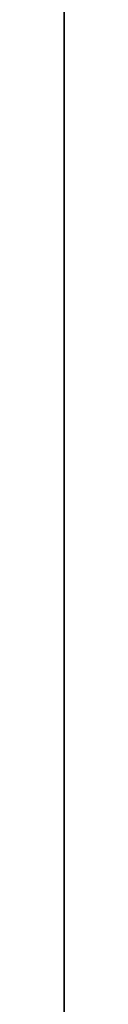
# Model space of a CAD drawing. Units: inches. Extents: x 2083 to 3317, y 1141 to 2115.
# Tile 67 of 256: x 2235.96 to 2235.96, y 1479.275 to 1481.434. Entities that reach past the tile are written whole.
import ezdxf

# ---------------------------------------------------------------- set-up
doc = ezdxf.new("R2010")
doc.units = ezdxf.units.IN
doc.layers.add('A-ANNO-DIMS', color=2, linetype='Continuous', lineweight=18)
doc.layers.add('A-WALL', color=7, linetype='Continuous', lineweight=35)
doc.layers.add('A-WALL-PATT', color=251, linetype='Continuous', lineweight=13, true_color=0x636466)
doc.styles.get("Standard").update_dxf_attribs({"font": 'arial.ttf'})
doc.dimstyles.new('ISO-25', dxfattribs={"dimtxt": 12, "dimasz": 12, "dimexe": 1.25, "dimexo": 0.625, "dimtad": 1, "dimlunit": 3, "dimtxsty": 'Standard', "dimcen": 2.5, "dimadec": 0, "dimazin": 0, "dimtfac": 1, "dimtmove": 0, "dimatfit": 3, "dimfxl": 1, "dimarcsym": 0})

# ---------------------------------------------------------------- blocks, each defined once
blk = doc.blocks.new('*D30')
at = {"layer": 'A-ANNO-DIMS', "color": 0, "lineweight": -2, "transparency": 16777216}
for p, q in [((2240.0179, 1445.2738), (2240.0179, 1448.0455)), ((2254.3293, 1445.2738), (2254.3293, 1448.0455)), ((2228.0179, 1446.7955), (2216.0179, 1446.7955)), ((2240.0179, 1446.7955), (2254.3293, 1446.7955)), ((2266.3293, 1446.7955), (2413.7649, 1446.7955))]:
    blk.add_line(p, q, dxfattribs=at)
at = {"layer": 'A-ANNO-DIMS', "color": 0, "transparency": 16777216}
for points in [[(2228.0179, 1448.7955), (2228.0179, 1444.7955), (2240.0179, 1446.7955)], [(2266.3293, 1448.7955), (2266.3293, 1444.7955), (2254.3293, 1446.7955)]]:
    blk.add_solid(points, dxfattribs=at)
at = {"layer": 'Defpoints', "color": 0, "transparency": 16777216}
for p in [(2254.3293, 1446.7955), (2240.0179, 1444.6488), (2254.3293, 1444.6488)]:
    blk.add_point(p, dxfattribs=at)
at = {"layer": 'A-ANNO-DIMS', "color": 0, "transparency": 16777216, "insert": (2346.0471, 1453.6252), "char_height": 12, "attachment_point": 5}
blk.add_mtext('WC 1\'-2 1/2" TYP.', dxfattribs=at)
blk = doc.blocks.new('*D31')
at = {"layer": 'A-ANNO-DIMS', "color": 0, "lineweight": -2, "transparency": 16777216}
for p, q in [((2237.8711, 1456.6488), (2237.8711, 1541.9152)), ((2239.3929, 1444.6488), (2236.6211, 1444.6488)), ((2237.8711, 1431.5475), (2237.8711, 1444.6488)), ((2239.3929, 1431.5475), (2236.6211, 1431.5475)), ((2237.8711, 1419.5475), (2237.8711, 1407.5475))]:
    blk.add_line(p, q, dxfattribs=at)
at = {"layer": 'A-ANNO-DIMS', "color": 0, "transparency": 16777216}
for points in [[(2235.8711, 1456.6488), (2239.8711, 1456.6488), (2237.8711, 1444.6488)], [(2235.8711, 1419.5475), (2239.8711, 1419.5475), (2237.8711, 1431.5475)]]:
    blk.add_solid(points, dxfattribs=at)
at = {"layer": 'Defpoints', "color": 0, "transparency": 16777216}
for p in [(2237.8711, 1444.6488), (2240.0179, 1444.6488), (2240.0179, 1431.5475)]:
    blk.add_point(p, dxfattribs=at)
at = {"layer": 'A-ANNO-DIMS', "color": 0, "transparency": 16777216, "insert": (2231.2175, 1505.282), "char_height": 12, "attachment_point": 5, "rotation": 90}
blk.add_mtext('1\'-1" TYP.', dxfattribs=at)
blk = doc.blocks.new('*D45')
at = {"layer": 'A-ANNO-DIMS', "color": 0, "lineweight": -2, "transparency": 16777216}
for p, q in [((2235.9598, 1478.3864), (2235.9598, 1531.3614)), ((2418.9598, 1478.3864), (2418.9598, 1531.3614)), ((2247.9598, 1530.1114), (2406.9598, 1530.1114))]:
    blk.add_line(p, q, dxfattribs=at)
at = {"layer": 'A-ANNO-DIMS', "color": 0, "transparency": 16777216}
for points in [[(2247.9598, 1532.1114), (2247.9598, 1528.1114), (2235.9598, 1530.1114)], [(2406.9598, 1532.1114), (2406.9598, 1528.1114), (2418.9598, 1530.1114)]]:
    blk.add_solid(points, dxfattribs=at)
at = {"layer": 'Defpoints', "color": 0, "transparency": 16777216}
for p in [(2418.9598, 1530.1114), (2235.9598, 1477.7614), (2418.9598, 1477.7614)]:
    blk.add_point(p, dxfattribs=at)
at = {"layer": 'A-ANNO-DIMS', "color": 0, "transparency": 16777216, "insert": (2327.4598, 1536.8673), "char_height": 12, "attachment_point": 5}
blk.add_mtext('15\'-3"', dxfattribs=at)
blk = doc.blocks.new('*D62')
at = {"layer": 'A-ANNO-DIMS', "color": 0, "lineweight": -2, "transparency": 16777216}
for p, q in [((2235.9598, 1469.3864), (2235.9598, 1522.3614)), ((2379.9598, 1469.3864), (2379.9598, 1522.3614)), ((2247.9598, 1521.1114), (2367.9598, 1521.1114))]:
    blk.add_line(p, q, dxfattribs=at)
at = {"layer": 'A-ANNO-DIMS', "color": 0, "transparency": 16777216}
for points in [[(2247.9598, 1523.1114), (2247.9598, 1519.1114), (2235.9598, 1521.1114)], [(2367.9598, 1523.1114), (2367.9598, 1519.1114), (2379.9598, 1521.1114)]]:
    blk.add_solid(points, dxfattribs=at)
at = {"layer": 'Defpoints', "color": 0, "transparency": 16777216}
for p in [(2379.9598, 1521.1114), (2235.9598, 1468.7614), (2379.9598, 1468.7614)]:
    blk.add_point(p, dxfattribs=at)
at = {"layer": 'A-ANNO-DIMS', "color": 0, "transparency": 16777216, "insert": (2307.9598, 1527.8632), "char_height": 12, "attachment_point": 5}
blk.add_mtext('12\'-0"', dxfattribs=at)

msp = doc.modelspace()

# ---------------------------------------------------------------- hatches: boundary and pattern name
at = {"layer": 'A-WALL-PATT'}
h = msp.add_hatch(color=256, dxfattribs=at)
h.dxf.hatch_style = 1
h.paths.add_polyline_path([(3126.9598, 2020.7614), (2748.9598, 2020.7614), (2604.9598, 2020.7614), (2226.9598, 2020.7614), (2226.9598, 1702.7614), (2466.9598, 1702.7614), (2466.9598, 1582.7614), (2418.9598, 1582.7614), (2418.9598, 1477.7614), (2226.9598, 1477.7614), (2226.9598, 1263.2614), (2544.9598, 1263.2614), (2544.9598, 1411.7614), (2604.9598, 1411.7614), (2685.9598, 1411.7614), (2685.9598, 1420.7614), (2604.9598, 1420.7614), (2604.9598, 1573.7614), (2604.9598, 1702.7614), (2604.9598, 2011.7614), (2748.9598, 2011.7614), (2748.9598, 1702.7614), (2862.9598, 1702.7614), (2862.9598, 1621.7614), (2871.9598, 1621.7614), (2871.9598, 1702.7614), (2883.9598, 1702.7614), (2883.9598, 1706.9395, -0.026459), (2883.9598, 1711.7614), (2757.9598, 1711.7614), (2757.9598, 1807.7614), (2787.9598, 1807.7614), (2787.9598, 1812.2614), (2757.9598, 1812.2614), (2757.9598, 2011.7614), (2877.9598, 2011.7614), (2877.9598, 1812.2614), (2847.9598, 1812.2614), (2847.9598, 1807.7614), (2889.8357, 1807.7614), (2889.8357, 1812.2614), (2882.4598, 1812.2614), (2882.4598, 2011.7614), (3117.9598, 2011.7614), (3117.9598, 1812.2614), (2937.8357, 1812.2614), (2937.8357, 1807.7614), (2995.7098, 1807.7614), (2995.7098, 1796.1177), (3000.2098, 1796.1177), (3000.2098, 1807.7614), (3117.9598, 1807.7614), (3117.9598, 1711.7614), (3000.2098, 1711.7614), (3000.2098, 1760.1177), (2998.5727, 1760.1177, -0.020711), (2995.7098, 1760.1177), (2995.7098, 1711.7614), (2931.9598, 1711.7614), (2931.9598, 1702.7614), (3126.9598, 1702.7614)])
h.paths.add_polyline_path([(2471.4598, 2011.7614), (2471.4598, 1810.0114), (2462.7169, 1810.0114), (2462.7169, 1805.5114), (2505.9598, 1805.5114), (2505.9598, 1810.0114), (2475.9598, 1810.0114), (2475.9598, 2011.7614), (2595.9598, 2011.7614), (2595.9598, 1810.0114), (2565.9598, 1810.0114), (2565.9598, 1805.5114), (2595.9598, 1805.5114), (2595.9598, 1711.7614), (2235.9598, 1711.7614), (2235.9598, 1805.5114), (2353.7098, 1805.5114), (2353.7098, 1796.0542), (2358.2098, 1796.0542), (2358.2098, 1805.5114), (2414.7169, 1805.5114), (2414.7169, 1810.0114), (2235.9598, 1810.0114), (2235.9598, 2011.7614)], flags=16)
h.paths.add_polyline_path([(2270.2047, 1994.61), (2270.2047, 1970.61), (2246.2047, 1970.61), (2246.2047, 1994.61)], flags=0)
edge = h.paths.add_edge_path(flags=0)
edge.add_ellipse((2332.0274, 1899.7982), major_axis=(-3.043, 3.043), ratio=0.168252, start_angle=-161.3322, end_angle=-156.3071, ccw=False)
edge.add_ellipse((2333.082, 1898.7435), major_axis=(-1.0546, 1.0546), ratio=0.453532, start_angle=-123.371, end_angle=-94.1591)
edge = h.paths.add_edge_path(flags=0)
edge.add_ellipse((2332.0274, 1968.8763), major_axis=(3.043, 3.043), ratio=0.168252, start_angle=18.6678, end_angle=23.6929)
edge.add_spline(control_points=[(2332.9256, 1970.6911), (2332.2268, 1970.3361), (2330.8937, 1969.6589), (2328.4131, 1970.9321), (2327.2039, 1967.7487), (2324.7096, 1969.9556), (2322.5328, 1967.0124), (2320.0128, 1971.2958), (2317.6803, 1968.1578), (2316.0405, 1967.102), (2315.4269, 1966.8096)], knot_values=[0, 0, 0, 0, 2.267059, 4.324559, 6.685584, 8.878641, 11.121502, 14.300359, 17.755284, 19.732645, 19.732645, 19.732645, 19.732645], degree=3, periodic=0)
edge.add_ellipse((2332.0274, 1968.8763), major_axis=(3.043, 3.043), ratio=0.168252, start_angle=18.6678, end_angle=23.6929, ccw=False)
edge.add_ellipse((2333.082, 1969.9309), major_axis=(1.0546, 1.0546), ratio=0.453532, start_angle=56.629, end_angle=85.8409, ccw=False)
edge = h.paths.add_edge_path(flags=0)
edge.add_spline(control_points=[(2296.4283, 1967.9879), (2293.6278, 1965.3363), (2287.7036, 1959.7271), (2299.7439, 1949.9957), (2294.5326, 1935.6685), (2290.5732, 1920.6035), (2293.3941, 1909.9737), (2296.1854, 1904.9665)], knot_values=[0.099185, 0.099185, 0.099185, 0.099185, 0.345301, 0.619822, 0.982653, 1.386093, 1.810555, 1.810555, 1.810555, 1.810555], degree=3, periodic=0)
edge.add_spline(control_points=[(2296.1854, 1904.9665), (2297.3836, 1902.6193), (2298.001, 1901.9493), (2298.553, 1901.4682)], knot_values=[0.006246, 0.006246, 0.006246, 0.006246, 0.055476, 0.055476, 0.055476, 0.055476], degree=3, periodic=0)
edge.add_spline(control_points=[(2298.553, 1901.4682), (2297.2586, 1900.9232), (2295.2253, 1900.2321), (2293.0602, 1900.6142), (2292.1014, 1900.7884), (2292.0896, 1900.7906)], knot_values=[0.312835, 0.312835, 0.312835, 0.312835, 0.40178, 0.474987, 0.475903, 0.475903, 0.475903, 0.475903], degree=3, periodic=0)
edge.add_arc((2292.7936, 1904.6641), 3.937, 215.4209, 259.6982, ccw=False)
edge.add_spline(control_points=[(2289.5853, 1902.3823), (2289.4767, 1902.5351), (2289.3685, 1902.688), (2289.2609, 1902.8412)], knot_values=[0.102872, 0.102872, 0.102872, 0.102872, 0.116896, 0.116896, 0.116896, 0.116896], degree=3, periodic=0)
edge.add_spline(control_points=[(2289.2609, 1902.8412), (2288.6866, 1902.5502), (2287.64, 1902.0199), (2285.8813, 1901.874), (2283.853, 1901.5044), (2281.72, 1899.7105), (2278.467, 1899.4929), (2276.1571, 1901.8832), (2272.259, 1899.8041), (2267.7776, 1901.8432), (2262.2439, 1900.184), (2257.4149, 1901.7821), (2254.3184, 1900.7261), (2253.1783, 1900.3373)], knot_values=[0, 0, 0, 0, 1.907977, 3.477176, 5.261074, 7.972851, 11.680248, 13.717921, 16.939592, 22.789562, 27.502503, 33.595215, 37.145618, 37.145618, 37.145618, 37.145618], degree=3, periodic=0)
edge.add_line((2253.1783, 1900.3373), (2250.2442, 1902.8412))
edge.add_line((2250.2442, 1902.8412), (2250.2442, 1965.8333))
edge.add_line((2250.2442, 1965.8333), (2253.1783, 1968.3371))
edge.add_spline(control_points=[(2253.1783, 1968.3371), (2254.3184, 1967.9483), (2257.4149, 1966.8924), (2262.2439, 1968.4904), (2267.7776, 1966.8313), (2271.5267, 1968.5372), (2273.8759, 1967.8283), (2274.2067, 1967.7276)], knot_values=[0, 0, 0, 0, 0.09018, 0.244935, 0.364644, 0.513233, 0.537855, 0.537855, 0.537855, 0.537855], degree=3, periodic=0)
edge.add_arc((2274.3529, 1963.7933), 3.937, 72.0511, 92.1279, ccw=False)
edge.add_arc((2281.2969, 1985.23), 18.5963, 252.05113, 288.56572)
edge.add_arc((2292.3167, 1956.0289), 12.6461, 71.02679, 113.77822, ccw=False)
edge = h.paths.add_edge_path(flags=0)
edge.add_spline(control_points=[(2274.8994, 1951.8562), (2275.0662, 1951.6166), (2275.2327, 1951.3766), (2275.398, 1951.1359)], knot_values=[1.409916, 1.409916, 1.409916, 1.409916, 1.43159, 1.43159, 1.43159, 1.43159], degree=3, periodic=0)
edge.add_spline(control_points=[(2275.398, 1951.1359), (2275.7921, 1950.5619), (2276.1792, 1949.9838), (2276.5455, 1949.3971)], knot_values=[1.358238, 1.358238, 1.358238, 1.358238, 1.409916, 1.409916, 1.409916, 1.409916], degree=3, periodic=0)
edge.add_line((2276.5455, 1949.3971), (2277.4373, 1947.8622))
edge.add_spline(control_points=[(2277.4373, 1947.8622), (2276.3038, 1945.6731), (2274.6397, 1942.4269), (2274.6316, 1938.0939), (2272.7991, 1930.8515), (2274.3564, 1943.897), (2275.9477, 1947.9234), (2276.5455, 1949.3971)], knot_values=[0.005632, 0.005632, 0.005632, 0.005632, 0.186014, 0.266002, 0.357087, 0.59639, 0.739732, 0.739732, 0.739732, 0.739732], degree=3, periodic=0)
edge.add_spline(control_points=[(2276.5455, 1949.3971), (2276.1792, 1949.9838), (2275.7921, 1950.5619), (2275.398, 1951.1359)], knot_values=[1.358238, 1.358238, 1.358238, 1.358238, 1.409916, 1.409916, 1.409916, 1.409916], degree=3, periodic=0)
edge.add_spline(control_points=[(2275.398, 1951.1359), (2274.9425, 1950.0805), (2274.2078, 1948.0253), (2273.9346, 1944.8515), (2272.4685, 1937.6275), (2273.4662, 1945.6965), (2274.7006, 1951.0595), (2274.8994, 1951.8562)], knot_values=[0.104364, 0.104364, 0.104364, 0.104364, 0.189636, 0.269624, 0.36071, 0.600013, 0.644622, 0.644622, 0.644622, 0.644622], degree=3, periodic=0)
h.paths.add_polyline_path([(2269.1675, 1963.1276, -0.357527), (2268.1706, 1960.9764, -0.092561), (2268.1706, 1939.4363, -0.357527), (2269.1675, 1937.2851, -0.357527), (2267.0163, 1938.282, -0.164785), (2254.6856, 1938.282, -0.357527), (2252.5344, 1937.2851, -0.357527), (2253.5313, 1939.4363, -0.092561), (2253.5313, 1960.9764, -0.357527), (2252.5344, 1963.1276, -0.357527), (2254.6856, 1962.1307, -0.164785), (2267.0163, 1962.1307, -0.357527)], flags=0)
h.paths.add_polyline_path([(2248.8741, 1967.8018), (2248.8741, 1957.0277), (2249.4578, 1957.0277), (2249.4578, 1911.6468), (2248.8741, 1911.6468), (2248.8741, 1900.8727), (2246.5119, 1900.8727, 0.197327), (2244.1497, 1902.4569), (2244.1497, 1966.2176, 0.197327), (2246.5119, 1967.8018)], flags=0)
h.paths.add_polyline_path([(2269.1675, 1931.3893, -0.357527), (2268.1706, 1929.2381, -0.092561), (2268.1706, 1907.6981, -0.357527), (2269.1675, 1905.5469, -0.357527), (2267.0163, 1906.5438, -0.164785), (2254.6856, 1906.5438, -0.357527), (2252.5344, 1905.5469, -0.357527), (2253.5313, 1907.6981, -0.092561), (2253.5313, 1929.2381, -0.357527), (2252.5344, 1931.3893, -0.357527), (2254.6856, 1930.3925, -0.164785), (2267.0163, 1930.3925, -0.357527)], flags=0)
edge = h.paths.add_edge_path(flags=0)
edge.add_spline(control_points=[(2276.1969, 1906.7237), (2276.1681, 1909.0289), (2276.114, 1913.3719), (2270.5984, 1924.925), (2273.9052, 1919.0128), (2275.9217, 1916.2621), (2275.4746, 1912.4021), (2277.2579, 1910.3806), (2276.696, 1908.225), (2276.6462, 1906.813), (2276.6178, 1906.0084)], knot_values=[0, 0, 0, 0, 8.61026, 16.221274, 18.843057, 23.804898, 27.440828, 29.356102, 31.203478, 33.650687, 33.650687, 33.650687, 33.650687], degree=3, periodic=0)
edge.add_spline(control_points=[(2276.6178, 1906.0084), (2276.6233, 1905.6241), (2276.4977, 1904.6287), (2275.4418, 1903.8547), (2274.9373, 1903.0804), (2274.8591, 1902.8412)], knot_values=[0.156488, 0.156488, 0.156488, 0.156488, 0.184398, 0.231376, 0.250598, 0.250598, 0.250598, 0.250598], degree=3, periodic=0)
edge.add_line((2274.8591, 1902.8412), (2276.506, 1902.8412))
edge.add_spline(control_points=[(2276.506, 1902.8412), (2276.7883, 1903.0849), (2277.6651, 1904.1252), (2278.2495, 1904.3407), (2277.6539, 1908.5274), (2278.1557, 1906.2278), (2278.1005, 1905.2859), (2278.8467, 1904.069), (2277.8568, 1903.4149), (2277.8742, 1902.991), (2277.9036, 1902.8412)], knot_values=[0.059574, 0.059574, 0.059574, 0.059574, 0.080753, 0.103741, 0.16972, 0.176036, 0.207137, 0.240474, 0.262341, 0.27366, 0.27366, 0.27366, 0.27366], degree=3, periodic=0)
edge.add_line((2277.9036, 1902.8412), (2280.0298, 1902.8412))
edge.add_spline(control_points=[(2280.0298, 1902.8412), (2279.8882, 1903.0884), (2279.4993, 1903.9816), (2280.1523, 1905.9393), (2278.1036, 1909.6578), (2279.7624, 1907.1853), (2280.3279, 1904.8749), (2280.4851, 1903.4896), (2281.4633, 1903.2494), (2281.7583, 1902.9365), (2281.834, 1902.8412)], knot_values=[0.013856, 0.013856, 0.013856, 0.013856, 0.034874, 0.088867, 0.107879, 0.126738, 0.158714, 0.193757, 0.217487, 0.226722, 0.226722, 0.226722, 0.226722], degree=3, periodic=0)
edge.add_spline(control_points=[(2281.834, 1902.8412), (2281.7875, 1902.8267), (2281.647, 1902.783), (2281.3955, 1902.8595), (2281.0881, 1902.9852), (2280.7207, 1903.0609), (2280.3335, 1903.0257), (2280.1248, 1902.8989), (2280.0298, 1902.8412)], knot_values=[0, 0, 0, 0, 0.14413, 0.435517, 0.749276, 1.153046, 1.548371, 1.878348, 1.878348, 1.878348, 1.878348], degree=3, periodic=0)
edge.add_line((2280.0298, 1902.8412), (2277.9036, 1902.8412))
edge.add_spline(control_points=[(2277.9036, 1902.8412), (2277.8929, 1902.7959), (2277.8654, 1902.6796), (2277.6075, 1902.6875), (2277.2741, 1902.8007), (2276.8379, 1902.6198), (2276.5838, 1902.7893), (2276.506, 1902.8412)], knot_values=[0, 0, 0, 0, 0.127189, 0.326199, 0.628009, 1.24357, 1.515331, 1.515331, 1.515331, 1.515331], degree=3, periodic=0)
edge.add_line((2276.506, 1902.8412), (2274.8591, 1902.8412))
edge.add_spline(control_points=[(2274.8591, 1902.8412), (2274.8144, 1902.8986), (2274.7251, 1903.0134), (2274.4935, 1903.119), (2274.2443, 1902.9605), (2273.9371, 1903.1849), (2273.614, 1902.9831), (2273.4083, 1902.883), (2273.3223, 1902.8412)], knot_values=[0, 0, 0, 0, 0.21843, 0.436957, 0.687977, 0.990379, 1.398396, 1.69185, 1.69185, 1.69185, 1.69185], degree=3, periodic=0)
edge.add_spline(control_points=[(2273.3223, 1902.8412), (2273.6167, 1903.4457), (2274.274, 1904.5383), (2276.0272, 1904.5737), (2276.207, 1906.5836), (2276.1969, 1906.7237)], knot_values=[0.012227, 0.012227, 0.012227, 0.012227, 0.059472, 0.106218, 0.134458, 0.134458, 0.134458, 0.134458], degree=3, periodic=0)
h.paths.add_polyline_path([(2270.7761, 1897.7898), (2270.7761, 1873.7898), (2246.7761, 1873.7898), (2246.7761, 1897.7898)], flags=0)
h.paths.add_polyline_path([(2353.7098, 1760.0051), (2353.7098, 1760.0542), (2358.2098, 1760.0542, -0.033729)], flags=0)
h.paths.add_polyline_path([(2321.8191, 1737.5292), (2341.9953, 1737.5292, -0.414214), (2343.2033, 1736.3212), (2343.2033, 1721.0206, -0.414214), (2341.9953, 1719.8127), (2321.8191, 1719.8127, -0.414214), (2320.6112, 1721.0206), (2320.6112, 1736.3212, -0.414214)], flags=0)
h.paths.add_polyline_path([(2324.235, 1736.3212), (2339.5794, 1736.3212, -0.414214), (2341.9953, 1733.9053), (2341.9953, 1725.4497, -0.414214), (2339.5794, 1723.0338), (2333.6806, 1723.0338), (2333.8453, 1722.0455, -0.870646), (2335.4254, 1721.8259, -0.767327), (2333.9227, 1721.4232), (2331.291, 1721.4232, -0.767327), (2329.7883, 1721.8259, -0.870646), (2331.3684, 1722.0455), (2331.5331, 1723.0338), (2324.235, 1723.0338, -0.414214), (2321.8191, 1725.4497), (2321.8191, 1733.9053, -0.414214)], flags=0)
h.paths.add_polyline_path([(2570.4838, 1928.6154), (2589.6838, 1928.6154), (2590.1688, 1928.6154), (2590.1688, 1904.9934), (2570.4838, 1904.9934)], flags=0)
h.paths.add_polyline_path([(2574.4473, 1927.2638, -1), (2572.8288, 1927.2638, -1)], flags=0)
h.paths.add_polyline_path([(2573.0899, 1926.9409), (2573.925, 1927.776), (2574.1477, 1927.5533), (2573.3126, 1926.7182)], flags=0)
h.paths.add_polyline_path([(2578.7791, 1919.7296, -1), (2571.5917, 1919.7296, -1)], flags=0)
h.paths.add_polyline_path([(2578.3854, 1919.7296, -1), (2571.9854, 1919.7296, -1)], flags=0)
h.paths.add_polyline_path([(2331.5958, 1729.4762, -1), (2333.618, 1729.4762, -1)], flags=0)
h.paths.add_polyline_path([(2578.0342, 1927.2638, -1), (2576.4157, 1927.2638, -1)], flags=0)
h.paths.add_polyline_path([(2576.6889, 1927.5311), (2576.9116, 1927.7538), (2577.7467, 1926.9186), (2577.524, 1926.6959)], flags=0)
h.paths.add_polyline_path([(2578.1391, 1909.8595, -1), (2572.2317, 1909.8595, -1)], flags=0)
h.paths.add_polyline_path([(2577.7454, 1909.8595, -1), (2572.6254, 1909.8595, -1)], flags=0)
h.paths.add_polyline_path([(2583.7977, 1927.2638, -1), (2582.1792, 1927.2638, -1)], flags=0)
h.paths.add_polyline_path([(2582.7186, 1927.7538), (2583.5538, 1926.9186), (2583.3311, 1926.6959), (2582.4959, 1927.5311)], flags=0)
h.paths.add_polyline_path([(2582.4959, 1927.5311), (2582.7186, 1927.7538), (2583.5538, 1926.9186), (2583.3311, 1926.6959)], flags=0)
h.paths.add_polyline_path([(2587.7391, 1920.5296, -1), (2581.8317, 1920.5296, -1)], flags=0)
h.paths.add_polyline_path([(2587.3454, 1920.5296, -1), (2582.2254, 1920.5296, -1)], flags=0)
h.paths.add_polyline_path([(2587.3846, 1927.2638, -1), (2585.7661, 1927.2638, -1)], flags=0)
h.paths.add_polyline_path([(2586.082, 1926.9802), (2586.9172, 1927.8154), (2587.1399, 1927.5927), (2586.3047, 1926.7575)], flags=0)
h.paths.add_polyline_path([(2588.3791, 1910.6595, -1), (2581.1917, 1910.6595, -1)], flags=0)
h.paths.add_polyline_path([(2587.9854, 1910.6595, -1), (2581.5854, 1910.6595, -1)], flags=0)
h.paths.add_polyline_path([(2417.1677, 1729.4779), (2437.3439, 1729.4779, -0.414214), (2438.5519, 1728.2699), (2438.5519, 1712.9693, -0.414214), (2437.3439, 1711.7614), (2417.1677, 1711.7614, -0.414214), (2415.9598, 1712.9693), (2415.9598, 1728.2699, -0.414214)], flags=0)
h.paths.add_polyline_path([(2419.5836, 1728.2699), (2434.928, 1728.2699, -0.414214), (2437.3439, 1725.8541), (2437.3439, 1717.3984, -0.414214), (2434.928, 1714.9825), (2429.0292, 1714.9825), (2429.1939, 1713.9942, -0.870646), (2430.774, 1713.7746, -0.767327), (2429.2713, 1713.372), (2426.6396, 1713.372, -0.767327), (2425.1369, 1713.7746, -0.870646), (2426.717, 1713.9942), (2426.8817, 1714.9825), (2419.5836, 1714.9825, -0.414214), (2417.1677, 1717.3984), (2417.1677, 1725.8541, -0.414214)], flags=0)
h.paths.add_polyline_path([(2419.5836, 1728.2699), (2434.928, 1728.2699, -0.414214), (2437.3439, 1725.8541), (2437.3439, 1717.3984, -0.414214), (2434.928, 1714.9825), (2429.0292, 1714.9825), (2428.3581, 1719.009), (2427.5528, 1719.009), (2426.8817, 1714.9825), (2419.5836, 1714.9825, -0.414214), (2417.1677, 1717.3984), (2417.1677, 1725.8541, -0.414214)], flags=0)
h.paths.add_polyline_path([(2426.9444, 1721.4249, -1), (2428.9666, 1721.4249, -1)], flags=0)
h.paths.add_polyline_path([(2475.9598, 1702.7614), (2595.9598, 1702.7614), (2595.9598, 1582.7614), (2475.9598, 1582.7614)], flags=16)
h.paths.add_polyline_path([(2427.9598, 1573.7614), (2595.9598, 1573.7614), (2595.9598, 1468.7614), (2595.9598, 1420.7614), (2384.4598, 1420.7614), (2384.4598, 1468.7614), (2427.9598, 1468.7614)], flags=16)
h.paths.add_polyline_path([(2379.9598, 1468.7614), (2379.9598, 1420.7614), (2235.9598, 1420.7614), (2235.9598, 1468.7614)], flags=16)
h.paths.add_polyline_path([(2317.816, 1466.6958), (2337.9922, 1466.6958, -0.414214), (2339.2002, 1465.4878), (2339.2002, 1450.1872, -0.414214), (2337.9922, 1448.9792), (2317.816, 1448.9792, -0.414214), (2316.6081, 1450.1872), (2316.6081, 1465.4878, -0.414214)], flags=0)
h.paths.add_polyline_path([(2320.2319, 1465.4878), (2335.5763, 1465.4878, -0.414214), (2337.9922, 1463.0719), (2337.9922, 1454.6163, -0.414214), (2335.5763, 1452.2004), (2329.6775, 1452.2004), (2329.8422, 1451.212, -0.870646), (2331.4223, 1450.9925, -0.767327), (2329.9196, 1450.5898), (2327.2879, 1450.5898, -0.767327), (2325.7852, 1450.9925, -0.870646), (2327.3653, 1451.212), (2327.53, 1452.2004), (2320.2319, 1452.2004, -0.414214), (2317.816, 1454.6163), (2317.816, 1463.0719, -0.414214)], flags=0)
h.paths.add_polyline_path([(2320.2319, 1465.4878), (2335.5763, 1465.4878, -0.414214), (2337.9922, 1463.0719), (2337.9922, 1454.6163, -0.414214), (2335.5763, 1452.2004), (2329.6775, 1452.2004), (2329.0064, 1456.2269), (2328.2011, 1456.2269), (2327.53, 1452.2004), (2320.2319, 1452.2004, -0.414214), (2317.816, 1454.6163), (2317.816, 1463.0719, -0.414214)], flags=0)
h.paths.add_polyline_path([(2327.5926, 1458.6428, -1), (2329.6148, 1458.6428, -1)], flags=0)
h.paths.add_polyline_path([(2244.4117, 1433.3405), (2241.9209, 1433.3405, -0.414214), (2240.0179, 1435.2435), (2240.0179, 1440.9528, -0.414211), (2241.9209, 1442.8559), (2244.4117, 1442.8559, -1.976472)], flags=0)
h.paths.add_polyline_path([(2245.3569, 1434.3975, -0.414214), (2245.3569, 1441.7988, -2.144098)], flags=0)
h.paths.add_polyline_path([(2535.9598, 1416.2614), (2535.9598, 1272.2614), (2235.9598, 1272.2614), (2235.9598, 1416.2614)], flags=16)
h.paths.add_polyline_path([(2260.1196, 1384.2928), (2260.1196, 1362.0386), (2237.8654, 1362.0386), (2237.8654, 1384.2928)], flags=0)
edge = h.paths.add_edge_path(flags=0)
edge.add_line((2318.2518, 1362.0933), (2318.1458, 1362.001))
edge.add_ellipse((2317.4451, 1360.431), major_axis=(2.8216, 2.8216), ratio=0.168252, start_angle=18.6678, end_angle=20.9481, ccw=False)
edge.add_ellipse((2318.423, 1361.409), major_axis=(0.9779, 0.9779), ratio=0.453532, start_angle=56.629, end_angle=70.2262, ccw=False)
edge = h.paths.add_edge_path(flags=0)
edge.add_line((2319.1074, 1295.5711), (2319.015, 1295.6771))
edge.add_ellipse((2317.4451, 1296.3778), major_axis=(-2.8216, 2.8216), ratio=0.168252, start_angle=-161.3322, end_angle=-159.0519, ccw=False)
edge.add_ellipse((2318.423, 1295.3999), major_axis=(-0.9779, 0.9779), ratio=0.453532, start_angle=-123.371, end_angle=-109.7738)
edge = h.paths.add_edge_path(flags=0)
edge.add_spline(control_points=[(2284.2103, 1301.1702), (2284.5807, 1300.4447), (2284.8912, 1299.892), (2285.1596, 1299.461)], knot_values=[0.039066, 0.039066, 0.039066, 0.039066, 0.055476, 0.055476, 0.055476, 0.055476], degree=3, periodic=0)
edge.add_line((2285.1596, 1299.461), (2284.2103, 1301.1702))
edge = h.paths.add_edge_path(flags=0)
edge.add_line((2280.4125, 1297.298), (2283.37, 1297.0361))
edge.add_line((2283.37, 1297.0361), (2286.4057, 1297.9263))
edge.add_spline(control_points=[(2286.4057, 1297.9263), (2285.3055, 1297.4631), (2284.3448, 1297.1292), (2283.37, 1297.0361)], knot_values=[0.394369, 0.394369, 0.394369, 0.394369, 0.475903, 0.475903, 0.475903, 0.475903], degree=3, periodic=0)
edge.add_spline(control_points=[(2283.37, 1297.0361), (2283.2814, 1297.0277), (2282.3163, 1296.9573), (2281.3125, 1297.1345), (2280.4234, 1297.296), (2280.4125, 1297.298)], knot_values=[0.312835, 0.312835, 0.312835, 0.312835, 0.320246, 0.393453, 0.394369, 0.394369, 0.394369, 0.394369], degree=3, periodic=0)
edge = h.paths.add_edge_path(flags=0)
edge.add_line((2284.4356, 1359.6073), (2280.4463, 1355.328))
edge.add_line((2280.4463, 1355.328), (2279.58, 1351.0178))
edge.add_line((2279.58, 1351.0178), (2282.413, 1346.5804))
edge.add_spline(control_points=[(2282.413, 1346.5804), (2283.1533, 1345.5892), (2284.2529, 1344.0289), (2284.801, 1342.3872), (2284.9352, 1341.8055)], knot_values=[1.240098, 1.240098, 1.240098, 1.240098, 1.332892, 1.382712, 1.382712, 1.382712, 1.382712], degree=3, periodic=0)
edge.add_spline(control_points=[(2284.9352, 1341.8055), (2285.3191, 1340.1406), (2285.233, 1338.4092), (2284.9099, 1336.6541)], knot_values=[1.097484, 1.097484, 1.097484, 1.097484, 1.240098, 1.240098, 1.240098, 1.240098], degree=3, periodic=0)
edge.add_spline(control_points=[(2284.9099, 1336.6541), (2284.5868, 1334.899), (2284.0267, 1333.1203), (2283.4626, 1331.3606)], knot_values=[0.95487, 0.95487, 0.95487, 0.95487, 1.097484, 1.097484, 1.097484, 1.097484], degree=3, periodic=0)
edge.add_line((2283.4626, 1331.3606), (2281.8904, 1326.1534))
edge.add_line((2281.8904, 1326.1534), (2280.7563, 1321.0561))
edge.add_line((2280.7563, 1321.0561), (2280.2992, 1316.002))
edge.add_line((2280.2992, 1316.002), (2280.7159, 1310.9501))
edge.add_line((2280.7159, 1310.9501), (2282.0281, 1305.9721))
edge.add_line((2282.0281, 1305.9721), (2284.2103, 1301.1702))
edge.add_spline(control_points=[(2284.2103, 1301.1702), (2283.3407, 1302.7302), (2282.6119, 1304.3365), (2282.0281, 1305.9721)], knot_values=[0.099185, 0.099185, 0.099185, 0.099185, 0.241799, 0.241799, 0.241799, 0.241799], degree=3, periodic=0)
edge.add_spline(control_points=[(2282.0281, 1305.9721), (2281.4443, 1307.6078), (2281.0055, 1309.2728), (2280.7159, 1310.9501)], knot_values=[0.241799, 0.241799, 0.241799, 0.241799, 0.384413, 0.384413, 0.384413, 0.384413], degree=3, periodic=0)
edge.add_spline(control_points=[(2280.7159, 1310.9501), (2280.4332, 1312.5876), (2280.2894, 1314.277), (2280.2989, 1315.962), (2280.2992, 1316.002)], knot_values=[0.384413, 0.384413, 0.384413, 0.384413, 0.523647, 0.527028, 0.527028, 0.527028, 0.527028], degree=3, periodic=0)
edge.add_spline(control_points=[(2280.2992, 1316.002), (2280.3123, 1317.687), (2280.4779, 1319.3679), (2280.7563, 1321.0561)], knot_values=[0.527028, 0.527028, 0.527028, 0.527028, 0.669642, 0.669642, 0.669642, 0.669642], degree=3, periodic=0)
edge.add_spline(control_points=[(2280.7563, 1321.0561), (2281.0346, 1322.7443), (2281.4259, 1324.4396), (2281.8904, 1326.1534)], knot_values=[0.669642, 0.669642, 0.669642, 0.669642, 0.812256, 0.812256, 0.812256, 0.812256], degree=3, periodic=0)
edge.add_spline(control_points=[(2281.8904, 1326.1534), (2282.2644, 1327.5333), (2282.7879, 1329.2618), (2283.3528, 1331.0178), (2283.4626, 1331.3606)], knot_values=[0.812256, 0.812256, 0.812256, 0.812256, 0.927087, 0.95487, 0.95487, 0.95487, 0.95487], degree=3, periodic=0)
edge.add_line((2283.4626, 1331.3606), (2284.9099, 1336.6541))
edge.add_line((2284.9099, 1336.6541), (2284.9352, 1341.8055))
edge.add_line((2284.9352, 1341.8055), (2282.413, 1346.5804))
edge.add_spline(control_points=[(2282.413, 1346.5804), (2281.2751, 1348.1038), (2280.0784, 1349.5703), (2279.58, 1351.0178)], knot_values=[1.382712, 1.382712, 1.382712, 1.382712, 1.525326, 1.525326, 1.525326, 1.525326], degree=3, periodic=0)
edge.add_spline(control_points=[(2279.58, 1351.0178), (2279.4433, 1351.4147), (2279.1363, 1352.8569), (2279.7352, 1354.2904), (2280.4463, 1355.328)], knot_values=[1.525326, 1.525326, 1.525326, 1.525326, 1.564439, 1.667941, 1.667941, 1.667941, 1.667941], degree=3, periodic=0)
edge.add_spline(control_points=[(2280.4463, 1355.328), (2281.4261, 1356.7578), (2282.9308, 1358.1826), (2284.4356, 1359.6073)], knot_values=[1.667941, 1.667941, 1.667941, 1.667941, 1.810555, 1.810555, 1.810555, 1.810555], degree=3, periodic=0)
edge.add_arc((2280.6231, 1348.5182), 11.7262, 71.02679, 113.77822)
edge.add_arc((2270.4049, 1375.5952), 17.2436, 252.05113, 288.56572, ccw=False)
edge.add_arc((2263.966, 1355.7178), 3.6506, 72.0511, 92.1279)
edge.add_arc((2263.966, 1355.7178), 3.6506, 92.1279, 177.9851)
edge.add_spline(control_points=[(2260.3176, 1355.8462), (2260.2604, 1354.2207), (2260.5513, 1350.1865), (2262.9993, 1346.7663), (2264.4727, 1344.649)], knot_values=[1.43159, 1.43159, 1.43159, 1.43159, 1.564144, 1.770695, 1.770695, 1.770695, 1.770695], degree=3, periodic=0)
edge.add_line((2264.4727, 1344.649), (2264.9356, 1343.9825))
edge.add_spline(control_points=[(2263.801, 1340.2481), (2263.8432, 1340.5141), (2264.0672, 1341.7565), (2264.5127, 1343.0025), (2264.935, 1343.9811)], knot_values=[0.53657, 0.53657, 0.53657, 0.53657, 0.559349, 0.644622, 0.644622, 0.644622, 0.644622], degree=3, periodic=0)
edge.add_spline(control_points=[(2264.935, 1343.9811), (2265.1178, 1343.715), (2265.2989, 1343.4479), (2265.4768, 1343.1794)], knot_values=[1.384077, 1.384077, 1.384077, 1.384077, 1.409916, 1.409916, 1.409916, 1.409916], degree=3, periodic=0)
edge.add_spline(control_points=[(2265.4768, 1343.1794), (2265.6546, 1342.9108), (2265.8293, 1342.6408), (2265.9991, 1342.3688)], knot_values=[1.358238, 1.358238, 1.358238, 1.358238, 1.384077, 1.384077, 1.384077, 1.384077], degree=3, periodic=0)
edge.add_line((2265.9991, 1342.3688), (2266.826, 1340.9455))
edge.add_spline(control_points=[(2266.826, 1340.9455), (2268.8944, 1337.0897), (2271.3982, 1325.843), (2270.5162, 1310.5686), (2275.9194, 1301.8606), (2277.7895, 1299.1994)], knot_values=[0.116896, 0.116896, 0.116896, 0.116896, 0.472987, 1.050969, 1.313793, 1.313793, 1.313793, 1.313793], degree=3, periodic=0)
edge.add_spline(control_points=[(2277.7895, 1299.1994), (2277.8394, 1299.1285), (2277.8894, 1299.0575), (2277.9396, 1298.9866)], knot_values=[0.109884, 0.109884, 0.109884, 0.109884, 0.116896, 0.116896, 0.116896, 0.116896], degree=3, periodic=0)
edge.add_line((2277.9396, 1298.9866), (2277.7888, 1299.1991))
edge.add_spline(control_points=[(2277.7888, 1299.1991), (2277.2566, 1298.9294), (2276.2864, 1298.4379), (2275.0394, 1298.3344), (2274.3833, 1298.2389), (2274.2153, 1298.2093)], knot_values=[33.12187, 33.12187, 33.12187, 33.12187, 35.029056, 36.598255, 37.144827, 37.144827, 37.144827, 37.144827], degree=3, periodic=0)
edge.add_line((2274.2153, 1298.2093), (2273.0731, 1297.893))
edge.add_spline(control_points=[(2273.0731, 1297.893), (2272.3229, 1297.5798), (2271.0392, 1296.5105), (2269.2484, 1296.2261), (2268.4231, 1296.3747)], knot_values=[26.532584, 26.532584, 26.532584, 26.532584, 29.198919, 31.839101, 31.839101, 31.839101, 31.839101], degree=3, periodic=0)
edge.add_line((2268.4231, 1296.3747), (2263.8785, 1297.4575))
edge.add_spline(control_points=[(2263.8785, 1297.4575), (2263.5561, 1297.3594), (2261.8603, 1296.8387), (2260.2388, 1297.2824), (2258.9335, 1297.5165)], knot_values=[15.919551, 15.919551, 15.919551, 15.919551, 16.939592, 21.226067, 21.226067, 21.226067, 21.226067], degree=3, periodic=0)
edge.add_line((2258.9335, 1297.5165), (2254.0552, 1297.329))
edge.add_spline(control_points=[(2254.0552, 1297.329), (2253.7555, 1297.2958), (2252.1137, 1297.1652), (2250.4619, 1297.5442), (2249.1297, 1297.6679)], knot_values=[5.306517, 5.306517, 5.306517, 5.306517, 6.276435, 10.613034, 10.613034, 10.613034, 10.613034], degree=3, periodic=0)
edge.add_line((2249.1297, 1297.6679), (2244.3316, 1296.8778))
edge.add_line((2244.3316, 1296.8778), (2241.611, 1299.1994))
edge.add_line((2241.611, 1299.1994), (2241.611, 1357.6094))
edge.add_line((2241.611, 1357.6094), (2244.3316, 1359.9311))
edge.add_line((2244.3316, 1359.9311), (2252.7288, 1359.5427))
edge.add_spline(control_points=[(2252.7288, 1359.5427), (2252.8709, 1359.5464), (2253.3057, 1359.5482), (2253.7398, 1359.5143), (2254.0317, 1359.4824)], knot_values=[0.233291, 0.233291, 0.233291, 0.233291, 0.244935, 0.268927, 0.268927, 0.268927, 0.268927], degree=3, periodic=0)
edge.add_line((2254.0317, 1359.4824), (2259.5872, 1359.4164))
edge.add_spline(control_points=[(2259.5872, 1359.4164), (2260.6771, 1359.6285), (2262.0732, 1359.897), (2263.5237, 1359.4593), (2263.8304, 1359.366)], knot_values=[0.422516, 0.422516, 0.422516, 0.422516, 0.513233, 0.537855, 0.537855, 0.537855, 0.537855], degree=3, periodic=0)
edge.add_arc((2263.966, 1355.7178), 3.6506, 72.0511, 92.1279, ccw=False)
edge.add_arc((2270.4049, 1375.5952), 17.2436, 252.05113, 288.56572)
edge.add_arc((2280.6231, 1348.5182), 11.7262, 71.02679, 113.77822, ccw=False)
h.paths.add_polyline_path([(2240.3405, 1359.4347), (2240.3405, 1349.4444), (2240.8818, 1349.4444), (2240.8818, 1307.3645), (2240.3405, 1307.3645), (2240.3405, 1297.3741), (2238.1502, 1297.3741, 0.197327), (2235.9598, 1298.8431), (2235.9598, 1357.9657, 0.197327), (2238.1502, 1359.4347)], flags=0)
h.paths.add_polyline_path([(2259.1578, 1355.1005, -0.357527), (2258.2334, 1353.1058, -0.092561), (2258.2334, 1333.1326, -0.357527), (2259.1578, 1331.1379, -0.357527), (2257.1631, 1332.0622, -0.164785), (2245.7293, 1332.0622, -0.357527), (2243.7346, 1331.1379, -0.357527), (2244.6589, 1333.1326, -0.092561), (2244.6589, 1353.1058, -0.357527), (2243.7346, 1355.1005, -0.357527), (2245.7293, 1354.1761, -0.164785), (2257.1631, 1354.1761, -0.357527)], flags=0)
edge = h.paths.add_edge_path(flags=0)
edge.add_line((2265.9991, 1342.3688), (2266.826, 1340.9455))
edge.add_line((2266.826, 1340.9455), (2265.3076, 1337.8141))
edge.add_line((2265.3076, 1337.8141), (2264.3582, 1334.6529))
edge.add_line((2264.3582, 1334.6529), (2264.262, 1333.7997))
edge.add_spline(control_points=[(2264.262, 1333.7997), (2264.2084, 1333.1871), (2264.1621, 1332.3655), (2264.0071, 1331.4139), (2263.969, 1331.2018)], knot_values=[0.464444, 0.464444, 0.464444, 0.464444, 0.516691, 0.531608, 0.531608, 0.531608, 0.531608], degree=3, periodic=0)
edge.add_spline(control_points=[(2263.969, 1331.2018), (2263.7745, 1330.1189), (2263.4244, 1328.7908), (2263.2574, 1328.5307), (2263.234, 1328.5146)], knot_values=[0.372682, 0.372682, 0.372682, 0.372682, 0.44885, 0.464444, 0.464444, 0.464444, 0.464444], degree=3, periodic=0)
edge.add_spline(control_points=[(2263.234, 1328.5146), (2263.0964, 1328.4202), (2263.1312, 1329.3015), (2263.275, 1330.6157)], knot_values=[0.280919, 0.280919, 0.280919, 0.280919, 0.372682, 0.372682, 0.372682, 0.372682], degree=3, periodic=0)
edge.add_spline(control_points=[(2263.275, 1330.6157), (2263.4187, 1331.93), (2263.6715, 1333.6773), (2263.9699, 1335.315)], knot_values=[0.189157, 0.189157, 0.189157, 0.189157, 0.280919, 0.280919, 0.280919, 0.280919], degree=3, periodic=0)
edge.add_spline(control_points=[(2263.9699, 1335.315), (2264.1005, 1336.0322), (2264.4188, 1337.6219), (2264.7548, 1338.8644), (2264.9474, 1339.4911)], knot_values=[0.097394, 0.097394, 0.097394, 0.097394, 0.137578, 0.189157, 0.189157, 0.189157, 0.189157], degree=3, periodic=0)
edge.add_spline(control_points=[(2264.9474, 1339.4911), (2265.29, 1340.6061), (2265.6442, 1341.494), (2265.9991, 1342.3688)], knot_values=[0.005632, 0.005632, 0.005632, 0.005632, 0.097394, 0.097394, 0.097394, 0.097394], degree=3, periodic=0)
h.paths.add_polyline_path([(2259.1578, 1325.671, -0.357527), (2258.2334, 1323.6763, -0.092561), (2258.2334, 1303.7031, -0.357527), (2259.1578, 1301.7084, -0.357527), (2257.1631, 1302.6327, -0.164785), (2245.7293, 1302.6327, -0.357527), (2243.7346, 1301.7084, -0.357527), (2244.6589, 1303.7031, -0.092561), (2244.6589, 1323.6763, -0.357527), (2243.7346, 1325.671, -0.357527), (2245.7293, 1324.7466, -0.164785), (2257.1631, 1324.7466, -0.357527)], flags=0)
edge = h.paths.add_edge_path(flags=0)
edge.add_spline(control_points=[(2261.7089, 1317.3114), (2261.6795, 1317.4176), (2261.7619, 1317.3885), (2262.4907, 1316.0899), (2262.9622, 1315.3009)], knot_values=[14.955861, 14.955861, 14.955861, 14.955861, 16.221274, 18.694826, 18.694826, 18.694826, 18.694826], degree=3, periodic=0)
edge.add_spline(control_points=[(2262.9622, 1315.3009), (2262.9904, 1315.2536), (2263.7021, 1314.0674), (2264.349, 1313.1272), (2264.7301, 1312.1642)], knot_values=[18.694826, 18.694826, 18.694826, 18.694826, 18.843057, 22.433791, 22.433791, 22.433791, 22.433791], degree=3, periodic=0)
edge.add_spline(control_points=[(2264.7301, 1312.1642), (2264.8756, 1311.7964), (2265.1769, 1310.7698), (2265.1431, 1309.5593), (2265.2477, 1308.8242)], knot_values=[22.433791, 22.433791, 22.433791, 22.433791, 23.804898, 26.172756, 26.172756, 26.172756, 26.172756], degree=3, periodic=0)
edge.add_line((2265.2477, 1308.8242), (2265.8508, 1307.1719))
edge.add_spline(control_points=[(2265.8508, 1307.1719), (2266.065, 1306.8217), (2266.3844, 1306.3322), (2266.4244, 1305.7805), (2266.4204, 1305.6112)], knot_values=[28.062562, 28.062562, 28.062562, 28.062562, 29.356102, 29.911721, 29.911721, 29.911721, 29.911721], degree=3, periodic=0)
edge.add_spline(control_points=[(2266.4204, 1305.6112), (2266.4161, 1305.4326), (2266.394, 1305.25), (2266.3648, 1305.0659)], knot_values=[29.911721, 29.911721, 29.911721, 29.911721, 30.497837, 30.497837, 30.497837, 30.497837], degree=3, periodic=0)
edge.add_line((2266.3648, 1305.0659), (2266.0662, 1302.1363))
edge.add_spline(control_points=[(2266.0662, 1302.1363), (2266.0712, 1301.78), (2265.9981, 1301.2), (2265.6633, 1300.759), (2265.5089, 1300.5859)], knot_values=[0.156488, 0.156488, 0.156488, 0.156488, 0.184398, 0.203543, 0.203543, 0.203543, 0.203543], degree=3, periodic=0)
edge.add_line((2265.5089, 1300.5859), (2264.4353, 1299.1994))
edge.add_line((2264.4353, 1299.1994), (2265.9624, 1299.1994))
edge.add_line((2265.9624, 1299.1994), (2267.336, 1301.1753))
edge.add_line((2267.336, 1301.1753), (2267.3117, 1301.9862))
edge.add_spline(control_points=[(2267.3117, 1301.9862), (2267.2611, 1302.8624), (2267.1602, 1303.7371), (2267.2715, 1303.3259)], knot_values=[0.126229, 0.126229, 0.126229, 0.126229, 0.166617, 0.166617, 0.166617, 0.166617], degree=3, periodic=0)
edge.add_spline(control_points=[(2267.2715, 1303.3259), (2267.28, 1303.2943), (2267.3098, 1303.1754), (2267.3735, 1302.8836), (2267.4061, 1302.6828), (2267.4179, 1302.601)], knot_values=[0.166617, 0.166617, 0.166617, 0.166617, 0.16972, 0.176036, 0.180765, 0.180765, 0.180765, 0.180765], degree=3, periodic=0)
edge.add_spline(control_points=[(2267.7439, 1300.9875), (2267.6876, 1301.1509), (2267.4805, 1301.6567), (2267.4838, 1302.1448), (2267.4179, 1302.601)], knot_values=[0.180765, 0.180765, 0.180765, 0.180765, 0.193767, 0.220139, 0.220139, 0.220139, 0.220139], degree=3, periodic=0)
edge.add_line((2267.4179, 1302.601), (2267.7439, 1300.9875))
edge.add_spline(control_points=[(2267.7439, 1300.9875), (2267.832, 1300.7319), (2267.932, 1300.3099), (2267.5548, 1299.9745), (2267.4294, 1299.8292)], knot_values=[0.220139, 0.220139, 0.220139, 0.220139, 0.240474, 0.25489, 0.25489, 0.25489, 0.25489], degree=3, periodic=0)
edge.add_line((2267.4294, 1299.8292), (2267.2584, 1299.1994))
edge.add_line((2267.2584, 1299.1994), (2269.23, 1299.1994))
edge.add_spline(control_points=[(2269.23, 1299.1994), (2269.0987, 1299.4287), (2268.8428, 1300.0163), (2269.0116, 1300.9159), (2268.9468, 1301.6607)], knot_values=[0.013856, 0.013856, 0.013856, 0.013856, 0.034874, 0.067073, 0.067073, 0.067073, 0.067073], degree=3, periodic=0)
edge.add_line((2268.9468, 1301.6607), (2268.4316, 1303.6031))
edge.add_spline(control_points=[(2268.4316, 1303.6031), (2268.1756, 1304.1924), (2267.5962, 1305.2513), (2268.0407, 1304.6232), (2268.2514, 1304.2824)], knot_values=[0.090155, 0.090155, 0.090155, 0.090155, 0.107879, 0.120289, 0.120289, 0.120289, 0.120289], degree=3, periodic=0)
edge.add_spline(control_points=[(2268.2514, 1304.2824), (2268.3609, 1304.1053), (2269.0578, 1302.918), (2269.3827, 1301.5904), (2269.5214, 1300.7759), (2269.5752, 1300.5558)], knot_values=[0.120289, 0.120289, 0.120289, 0.120289, 0.126738, 0.158714, 0.173506, 0.173506, 0.173506, 0.173506], degree=3, periodic=0)
edge.add_line((2269.5752, 1300.5558), (2270.6858, 1299.4213))
edge.add_spline(control_points=[(2270.6858, 1299.4213), (2270.7672, 1299.3573), (2270.8379, 1299.2814), (2270.9029, 1299.1994)], knot_values=[0.21816, 0.21816, 0.21816, 0.21816, 0.226722, 0.226722, 0.226722, 0.226722], degree=3, periodic=0)
edge.add_line((2270.9372, 1299.1929), (2270.9029, 1299.1994))
edge.add_spline(control_points=[(2270.9029, 1299.1994), (2270.8598, 1299.186), (2270.7295, 1299.1455), (2270.4963, 1299.2164), (2270.2717, 1299.3083), (2270.121, 1299.348), (2270.0633, 1299.3596)], knot_values=[0.939174, 0.939174, 0.939174, 0.939174, 1.083304, 1.374691, 1.68845, 1.878348, 1.878348, 1.878348, 1.878348], degree=3, periodic=0)
edge.add_line((2270.0633, 1299.3596), (2269.23, 1299.1994))
edge.add_line((2269.23, 1299.1994), (2267.2584, 1299.1994))
edge.add_spline(control_points=[(2267.2584, 1299.1994), (2267.2484, 1299.1574), (2267.223, 1299.0497), (2266.9838, 1299.0569), (2266.8092, 1299.1162), (2266.6769, 1299.1091), (2266.6365, 1299.1048)], knot_values=[0.757665, 0.757665, 0.757665, 0.757665, 0.884854, 1.083864, 1.385675, 1.515331, 1.515331, 1.515331, 1.515331], degree=3, periodic=0)
edge.add_spline(control_points=[(2266.6365, 1299.1048), (2266.4852, 1299.0888), (2266.2358, 1299.0171), (2266.0346, 1299.1513), (2265.9624, 1299.1994)], knot_values=[0, 0, 0, 0, 0.485905, 0.757665, 0.757665, 0.757665, 0.757665], degree=3, periodic=0)
edge.add_line((2265.9624, 1299.1994), (2264.4353, 1299.1994))
edge.add_line((2264.4353, 1299.1994), (2263.8584, 1299.3671))
edge.add_spline(control_points=[(2263.8584, 1299.3671), (2263.8189, 1299.3709), (2263.7795, 1299.3857), (2263.7401, 1299.4015)], knot_values=[0.845925, 0.845925, 0.845925, 0.845925, 0.978627, 0.978627, 0.978627, 0.978627], degree=3, periodic=0)
edge.add_line((2263.7218, 1299.3964), (2263.0103, 1299.1994))
edge.add_spline(control_points=[(2263.0103, 1299.1994), (2263.2458, 1299.6829), (2263.506, 1300.1281), (2263.8735, 1300.408)], knot_values=[0.012227, 0.012227, 0.012227, 0.012227, 0.052971, 0.052971, 0.052971, 0.052971], degree=3, periodic=0)
edge.add_spline(control_points=[(2263.8735, 1300.408), (2263.9321, 1300.4527), (2264.0842, 1300.553), (2264.2552, 1300.6242), (2264.3597, 1300.6647)], knot_values=[0.052971, 0.052971, 0.052971, 0.052971, 0.059472, 0.069086, 0.069086, 0.069086, 0.069086], degree=3, periodic=0)
edge.add_line((2264.3597, 1300.6647), (2265.1419, 1301.0778))
edge.add_line((2265.1419, 1301.0778), (2265.6758, 1302.7996))
edge.add_line((2265.6758, 1302.7996), (2265.5407, 1305.7041))
edge.add_line((2265.5407, 1305.7041), (2264.8031, 1309.3277))
edge.add_line((2264.8031, 1309.3277), (2263.0405, 1314.0918))
edge.add_spline(control_points=[(2263.0405, 1314.0918), (2262.3836, 1315.6714), (2261.796, 1316.9977), (2261.7089, 1317.3114)], knot_values=[11.216896, 11.216896, 11.216896, 11.216896, 14.955861, 14.955861, 14.955861, 14.955861], degree=3, periodic=0)
h.paths.add_polyline_path([(2871.9598, 1416.2614), (2895.91, 1416.2614), (2895.91, 1420.7614), (2871.9598, 1420.7614), (2871.9598, 1501.7614), (2862.9598, 1501.7614), (2862.9598, 1420.7614), (2805.9598, 1420.7614), (2805.9598, 1411.7614), (2862.9598, 1411.7614), (2862.9598, 1263.2614), (3126.9598, 1263.2614), (3126.9598, 1411.7614), (3126.9598, 1486.7614), (2943.9598, 1486.7614), (2943.9598, 1477.7614), (2967.8603, 1477.7614), (2967.8603, 1420.7614), (2943.91, 1420.7614), (2943.91, 1416.2614), (3117.9598, 1416.2614), (3117.9598, 1420.7614), (2972.3603, 1420.7614), (2972.3603, 1477.7614), (3117.9598, 1477.7614), (3117.9598, 1420.7614), (3117.9598, 1272.2614), (2871.9598, 1272.2614)], flags=0)
h.paths.add_polyline_path([(2457.1256, 1485.9425), (2527.6027, 1485.9425), (2527.6027, 1537.6357), (2457.1256, 1537.6357)], flags=8)
h.paths.add_polyline_path([(2481.0051, 1609.9818), (2590.7658, 1609.9818), (2590.7658, 1682.0034), (2481.0051, 1682.0034)], flags=8)
h.paths.add_polyline_path([(2483.085, 1729.1268), (2553.562, 1729.1268), (2553.562, 1780.82), (2483.085, 1780.82)], flags=8)

# ---------------------------------------------------------------- linework, layer by layer
at = {"layer": 'A-WALL'}
msp.add_line((2235.9598, 1702.7614), (2235.9598, 1477.7614), dxfattribs=at)
msp.add_line((2235.9598, 1702.7614), (2235.9598, 1477.7614), dxfattribs=at)

# ---------------------------------------------------------------- dimensions: what is measured, and where the dimension line sits
at = {"layer": 'A-ANNO-DIMS'}
for base, p1, p2, picture, middle in [((2418.9598, 1530.1114), (2235.9598, 1477.7614), (2418.9598, 1477.7614), '*D45', (2327.4598, 1536.8673)), ((2379.9598, 1521.1114), (2235.9598, 1468.7614), (2379.9598, 1468.7614), '*D62', (2307.9598, 1527.8632))]:
    dim = msp.add_linear_dim(base=base, p1=p1, p2=p2, dimstyle='ISO-25', override={"dimdec": 1, "dimlfac": 1, "dimrnd": 0, "dimzin": 1, "dimdsep": 46, "dimlunit": 4, "dimfrac": 2}, dxfattribs=at)
    dim.commit()
    dim.dimension.update_dxf_attribs({"geometry": picture, "text_midpoint": middle})
dim = msp.add_linear_dim(base=(2237.8711, 1444.6488), p1=(2240.0179, 1431.5475), p2=(2240.0179, 1444.6488), angle=90, text='<> TYP.', dimstyle='ISO-25', override={"dimdec": 1, "dimlfac": 1, "dimrnd": 0, "dimzin": 1, "dimdsep": 46, "dimlunit": 4, "dimfrac": 2}, dxfattribs=at)
dim.commit()
dim.dimension.update_dxf_attribs({"geometry": '*D31', "text_midpoint": (2231.2175, 1505.282)})
dim = msp.add_linear_dim(base=(2254.3293, 1446.7955), p1=(2240.0179, 1444.6488), p2=(2254.3293, 1444.6488), text='WC <> TYP.', dimstyle='ISO-25', override={"dimdec": 1, "dimlfac": 1, "dimrnd": 0, "dimzin": 1, "dimdsep": 46, "dimlunit": 4, "dimfrac": 2}, dxfattribs=at)
dim.commit()
dim.dimension.update_dxf_attribs({"geometry": '*D30', "text_midpoint": (2346.0471, 1453.6252)})

doc.saveas('drawing.dxf')
